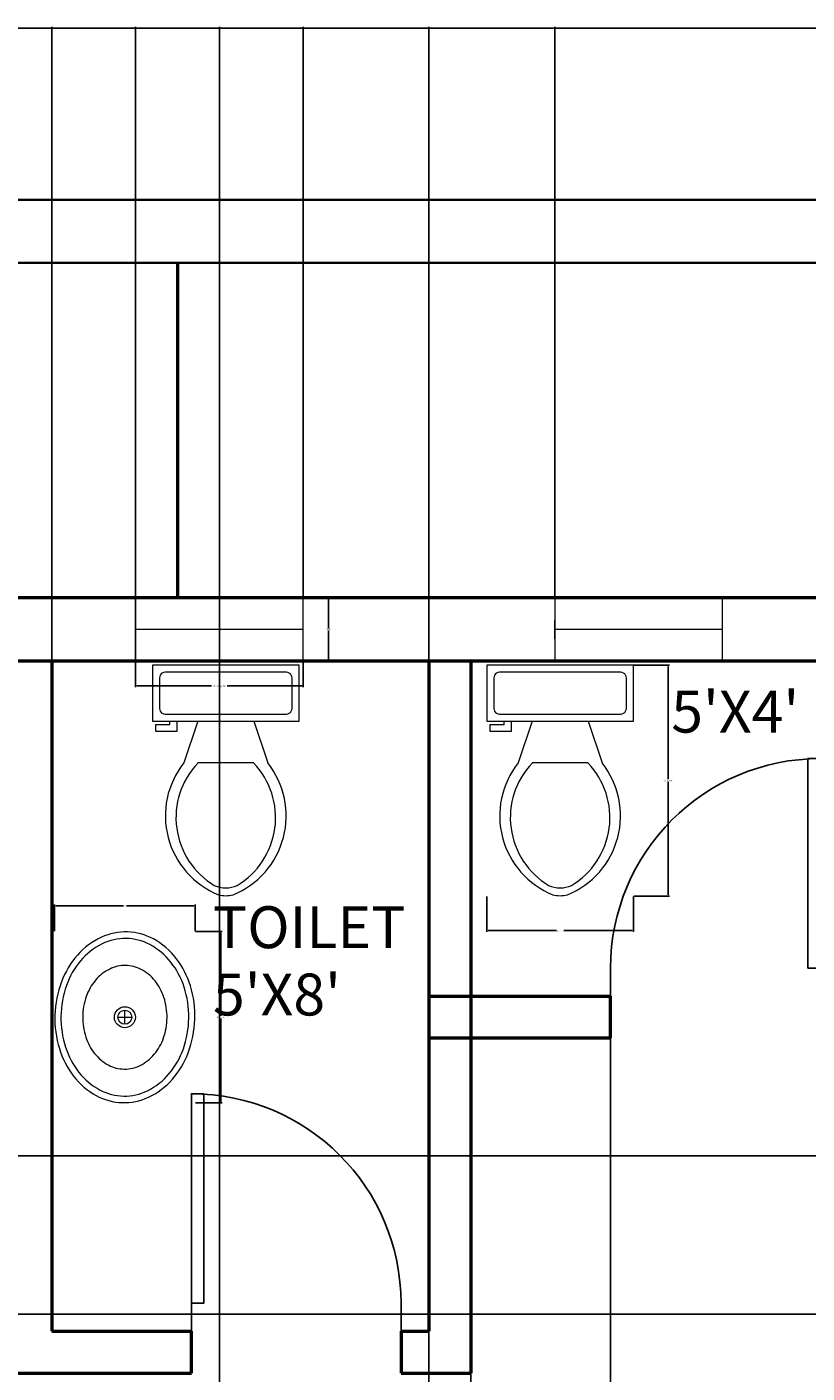
# Model space of a CAD drawing. Units: inches. Extents: x 8049 to 8459, y 820 to 1350.
# Tile 24 of 25: x 8182 to 8294, y 1157 to 1350. Entities that reach past the tile are written whole.
import ezdxf

# ---------------------------------------------------------------- set-up
doc = ezdxf.new("R2010")
doc.units = ezdxf.units.IN
doc.header["$MEASUREMENT"] = 0
for name, color, linetype, lineweight in [('A-ANNO-DIMS', 2, 'Continuous', 18), ('A-AREA-IDEN', 7, 'Continuous', 25), ('A-DOOR', 3, 'Continuous', 25), ('A-FLOR-FIXT', 9, 'Continuous', 18), ('A-GLAZ', 4, 'Continuous', 18), ('A-WALL', 7, 'Continuous', 50), ('C-SITE-WALL', 7, 'Continuous', 35)]:
    doc.layers.add(name, color=color, linetype=linetype, lineweight=lineweight)
doc.styles.get("Standard").update_dxf_attribs({"font": 'arial.ttf'})
doc.dimstyles.get("Standard").update_dxf_attribs({"dimtxt": 0.18, "dimasz": 0.18, "dimexe": 0.18, "dimexo": 0.0625, "dimgap": 0.09, "dimtad": 0, "dimtih": 1, "dimtoh": 1, "dimdec": 4, "dimzin": 0, "dimdsep": 46, "dimtxsty": 'Standard', "dimcen": 0.09, "dimadec": 0, "dimazin": 0, "dimtfac": 1, "dimtdec": 4, "dimtofl": 0, "dimtmove": 0, "dimatfit": 3, "dimfxl": 1, "dimtolj": 1, "dimtzin": 0, "dimarcsym": 0})

# ---------------------------------------------------------------- blocks, each defined once
blk = doc.blocks.new('*U2')
for p, q in [((0, 0), (0, -100)), ((750, 0), (750, -100))]:
    blk.add_line(p, q)
blk.add_lwpolyline([(0, 0), (0, 750), (43.75, 750), (43.75, 0)], close=True)
blk.add_arc((0, 0), 750, 0, 90)
blk = doc.blocks.new('*U4')
for p, q in [((0, 100), (0, 0)), ((900, 100), (900, 0)), ((0, 50), (900, 50))]:
    blk.add_line(p, q)
blk = doc.blocks.new('Sink - Oval top')
for p, q in [((-1, 0), (1, 0)), ((0, 1), (0, -1))]:
    blk.add_line(p, q)
for points in [[(-12.23, 0.39, 0.117634), (-11.46, -3.36, 0.104469), (-8.88, -6.8, 0.090016), (-5.08, -9.07, 0.08192), (-0.32, -10.02, 0.08192), (4.49, -9.38, 0.090016), (8.42, -7.36, 0.104469), (11.22, -4.09, 0.117634), (12.23, -0.39, 0.117634), (11.46, 3.36, 0.104469), (8.88, 6.8, 0.090016), (5.08, 9.07, 0.08192), (0.32, 10.02, 0.08192), (-4.49, 9.38, 0.090016), (-8.42, 7.36, 0.104469), (-11.22, 4.09, 0.117634)], [(-11.29, 0.16, 0.118622), (-10.52, -3.25, 0.104678), (-8.07, -6.36, 0.089562), (-4.54, -8.37, 0.081185), (-0.13, -9.15, 0.081185), (4.3, -8.49, 0.089562), (7.89, -6.58, 0.104678), (10.42, -3.55, 0.118622), (11.29, -0.16, 0.118622), (10.52, 3.25, 0.104678), (8.07, 6.36, 0.089562), (4.54, 8.37, 0.081185), (0.13, 9.15, 0.081185), (-4.3, 8.49, 0.089562), (-7.89, 6.58, 0.104678), (-10.42, 3.55, 0.118622)], [(-7.42, 0.08, 0.118283), (-6.91, -2.17, 0.104607), (-5.29, -4.21, 0.089718), (-2.97, -5.53, 0.081436), (-0.07, -6.04, 0.081436), (2.84, -5.59, 0.089718), (5.2, -4.33, 0.104607), (6.86, -2.32, 0.118283), (7.42, -0.08, 0.118283), (6.91, 2.17, 0.104607), (5.29, 4.21, 0.089718), (2.97, 5.53, 0.081436), (0.07, 6.04, 0.081436), (-2.84, 5.59, 0.089718), (-5.2, 4.33, 0.104607), (-6.86, 2.32, 0.118283)]]:
    blk.add_lwpolyline(points, format="xyb", close=True)
for radius in [1.5, 1]:
    blk.add_circle((0, 0), radius)
blk = doc.blocks.new('Toilet - top')
for p, q in [((9.5, -6), (9.5, -2)), ((-10, -8.5), (-8, -8.5)), ((-10, -9.5), (-10, -8.5)), ((-7, -9.5), (-10, -9.5)), ((-8, -8.5), (-8, -8)), ((-7, -8), (-7, -9.5)), ((-4, -8), (-6, -14)), ((4, -8), (6, -14)), ((4, -14), (-4, -14))]:
    blk.add_line(p, q)
blk.add_lwpolyline([(10.5, -8), (10.5, 0), (-10.5, 0), (-10.5, -8)], close=True)
for points in [[(8.5, -1), (-8.5, -1)], [(-9.5, -2), (-9.5, -6)], [(-8.5, -7), (8.5, -7)]]:
    blk.add_lwpolyline(points)
for centre, radius, start, end in [((-8.62, -1.88), 0.884, 81.8699, 188.1301), ((8.62, -1.88), 0.884, 351.8699, 98.1301), ((-8.62, -6.12), 0.884, 171.8699, 278.1301), ((8.62, -6.12), 0.884, 261.8699, 8.1301), ((3.52, -21.58), 12.17, 141.4691, 247.9714), ((4.2, -21.82), 11.33, 136.3677, 238.9468), ((-3.52, -21.58), 12.17, 292.0284, 38.5307), ((-4.2, -21.82), 11.33, 301.053, 43.6321), ((0, -27.88), 4, 245.7318, 294.2682), ((0, -29), 4, 254.8605, 285.1395)]:
    blk.add_arc(centre, radius, start, end)
blk = doc.blocks.new('WIN-24IN-SURROUND')
for p, q in [((24, 9), (0, 9)), ((0, 9), (0, 0)), ((24, 0), (24, 9))]:
    blk.add_line(p, q)
blk = doc.blocks.new('*D32')
at = {"layer": 'A-ANNO-DIMS', "color": 0, "lineweight": -2, "transparency": 16777216}
for p, q in [((8197.4, 1258.81), (8197.4, 1255.09)), ((8221.4, 1258.81), (8221.4, 1255.09)), ((8197.58, 1255.27), (8208.28, 1255.27)), ((8221.22, 1255.27), (8210.52, 1255.27))]:
    blk.add_line(p, q, dxfattribs=at)
at = {"layer": 'A-ANNO-DIMS', "color": 0, "transparency": 16777216}
for points in [[(8197.58, 1255.3), (8197.58, 1255.24), (8197.4, 1255.27)], [(8221.22, 1255.3), (8221.22, 1255.24), (8221.4, 1255.27)]]:
    blk.add_solid(points, dxfattribs=at)
at = {"layer": 'Defpoints', "color": 0, "transparency": 16777216}
for p in [(8197.4, 1258.87), (8221.4, 1258.87), (8221.4, 1255.27)]:
    blk.add_point(p, dxfattribs=at)
at = {"layer": 'A-ANNO-DIMS', "color": 0, "transparency": 16777216, "insert": (8209.4, 1255.27), "char_height": 0.18, "attachment_point": 5}
blk.add_mtext('\\A1;WINDOW 24 TYP.', dxfattribs=at)
blk = doc.blocks.new('*D33')
at = {"layer": 'A-ANNO-DIMS', "color": 0, "lineweight": -2, "transparency": 16777216}
for p, q in [((8221.46, 1267.87), (8225.18, 1267.87)), ((8225, 1267.69), (8225, 1263.55)), ((8225, 1259.05), (8225, 1263.19)), ((8221.46, 1258.87), (8225.18, 1258.87))]:
    blk.add_line(p, q, dxfattribs=at)
at = {"layer": 'A-ANNO-DIMS', "color": 0, "transparency": 16777216}
for points in [[(8224.97, 1267.69), (8225.03, 1267.69), (8225, 1267.87)], [(8224.97, 1259.05), (8225.03, 1259.05), (8225, 1258.87)]]:
    blk.add_solid(points, dxfattribs=at)
at = {"layer": 'Defpoints', "color": 0, "transparency": 16777216}
for p in [(8221.4, 1267.87), (8225, 1267.87), (8221.4, 1258.87)]:
    blk.add_point(p, dxfattribs=at)
at = {"layer": 'A-ANNO-DIMS', "color": 0, "transparency": 16777216, "insert": (8225, 1263.37), "char_height": 0.18, "attachment_point": 5}
blk.add_mtext('\\A1;9 TYP.', dxfattribs=at)
blk = doc.blocks.new('*D36')
at = {"layer": 'A-ANNO-DIMS', "color": 0, "lineweight": -2, "transparency": 16777216}
for p, q in [((8268.73, 1258.24), (8273.81, 1258.24)), ((8273.63, 1258.06), (8273.63, 1241.9)), ((8273.63, 1225.37), (8273.63, 1241.53)), ((8268.73, 1225.19), (8273.81, 1225.19))]:
    blk.add_line(p, q, dxfattribs=at)
at = {"layer": 'A-ANNO-DIMS', "color": 0, "transparency": 16777216}
for points in [[(8273.6, 1258.06), (8273.66, 1258.06), (8273.63, 1258.24)], [(8273.6, 1225.37), (8273.66, 1225.37), (8273.63, 1225.19)]]:
    blk.add_solid(points, dxfattribs=at)
at = {"layer": 'Defpoints', "color": 0, "transparency": 16777216}
for p in [(8268.67, 1258.24), (8273.63, 1258.24), (8268.67, 1225.19)]:
    blk.add_point(p, dxfattribs=at)
at = {"layer": 'A-ANNO-DIMS', "color": 0, "transparency": 16777216, "insert": (8273.63, 1241.72), "char_height": 0.18, "attachment_point": 5}
blk.add_mtext('\\A1;WC 33 TYP.', dxfattribs=at)
blk = doc.blocks.new('*D37')
at = {"layer": 'A-ANNO-DIMS', "color": 0, "lineweight": -2, "transparency": 16777216}
for p, q in [((8247.67, 1225.13), (8247.67, 1220.06)), ((8268.67, 1225.13), (8268.67, 1220.06)), ((8247.85, 1220.24), (8257.64, 1220.24)), ((8268.49, 1220.24), (8258.7, 1220.24))]:
    blk.add_line(p, q, dxfattribs=at)
at = {"layer": 'A-ANNO-DIMS', "color": 0, "transparency": 16777216}
for points in [[(8247.85, 1220.27), (8247.85, 1220.21), (8247.67, 1220.24)], [(8268.49, 1220.27), (8268.49, 1220.21), (8268.67, 1220.24)]]:
    blk.add_solid(points, dxfattribs=at)
at = {"layer": 'Defpoints', "color": 0, "transparency": 16777216}
for p in [(8247.67, 1225.19), (8268.67, 1225.19), (8268.67, 1220.24)]:
    blk.add_point(p, dxfattribs=at)
at = {"layer": 'A-ANNO-DIMS', "color": 0, "transparency": 16777216, "insert": (8258.17, 1220.24), "char_height": 0.18, "attachment_point": 5}
blk.add_mtext('\\A1;21 TYP.', dxfattribs=at)
blk = doc.blocks.new('*D44')
at = {"layer": 'A-ANNO-DIMS', "color": 0, "lineweight": -2, "transparency": 16777216}
for p, q in [((8205.99, 1220.1), (8209.79, 1220.1)), ((8209.61, 1219.92), (8209.61, 1208.01)), ((8209.61, 1195.73), (8209.61, 1207.64)), ((8205.99, 1195.55), (8209.79, 1195.55))]:
    blk.add_line(p, q, dxfattribs=at)
at = {"layer": 'A-ANNO-DIMS', "color": 0, "transparency": 16777216}
for points in [[(8209.58, 1219.92), (8209.64, 1219.92), (8209.61, 1220.1)], [(8209.58, 1195.73), (8209.64, 1195.73), (8209.61, 1195.55)]]:
    blk.add_solid(points, dxfattribs=at)
at = {"layer": 'Defpoints', "color": 0, "transparency": 16777216}
for p in [(8205.93, 1220.1), (8209.61, 1220.1), (8205.93, 1195.55)]:
    blk.add_point(p, dxfattribs=at)
at = {"layer": 'A-ANNO-DIMS', "color": 0, "transparency": 16777216, "insert": (8209.61, 1207.83), "char_height": 0.18, "attachment_point": 5}
blk.add_mtext('\\A1;BASIN 25', dxfattribs=at)
blk = doc.blocks.new('*D45')
at = {"layer": 'A-ANNO-DIMS', "color": 0, "lineweight": -2, "transparency": 16777216}
for p, q in [((8185.79, 1220.17), (8185.79, 1223.97)), ((8185.97, 1223.79), (8195.64, 1223.79)), ((8205.75, 1223.79), (8196.08, 1223.79)), ((8205.93, 1220.17), (8205.93, 1223.97))]:
    blk.add_line(p, q, dxfattribs=at)
at = {"layer": 'A-ANNO-DIMS', "color": 0, "transparency": 16777216}
for points in [[(8185.97, 1223.82), (8185.97, 1223.76), (8185.79, 1223.79)], [(8205.75, 1223.82), (8205.75, 1223.76), (8205.93, 1223.79)]]:
    blk.add_solid(points, dxfattribs=at)
at = {"layer": 'Defpoints', "color": 0, "transparency": 16777216}
for p in [(8185.79, 1223.79), (8185.79, 1220.1), (8205.93, 1220.1)]:
    blk.add_point(p, dxfattribs=at)
at = {"layer": 'A-ANNO-DIMS', "color": 0, "transparency": 16777216, "insert": (8195.86, 1223.79), "char_height": 0.18, "attachment_point": 5}
blk.add_mtext('\\A1;20', dxfattribs=at)
blk = doc.blocks.new('*D48')
at = {"layer": 'A-ANNO-DIMS', "color": 0, "lineweight": -2, "transparency": 16777216}
for p, q in [((8074.4, 1324.93), (8074.4, 1349.65)), ((8074.58, 1349.47), (8254.11, 1349.47)), ((8434.22, 1349.47), (8254.69, 1349.47)), ((8434.4, 1324.93), (8434.4, 1349.65))]:
    blk.add_line(p, q, dxfattribs=at)
at = {"layer": 'A-ANNO-DIMS', "color": 0, "transparency": 16777216}
for points in [[(8074.58, 1349.5), (8074.58, 1349.44), (8074.4, 1349.47)], [(8434.22, 1349.5), (8434.22, 1349.44), (8434.4, 1349.47)]]:
    blk.add_solid(points, dxfattribs=at)
at = {"layer": 'Defpoints', "color": 0, "transparency": 16777216}
for p in [(8434.4, 1349.47), (8074.4, 1324.87), (8434.4, 1324.87)]:
    blk.add_point(p, dxfattribs=at)
at = {"layer": 'A-ANNO-DIMS', "color": 0, "transparency": 16777216, "insert": (8254.4, 1349.47), "char_height": 0.18, "attachment_point": 5}
blk.add_mtext('\\A1;360', dxfattribs=at)
blk = doc.blocks.new('*D64')
at = {"layer": 'A-ANNO-DIMS', "color": 0, "lineweight": -2, "transparency": 16777216}
for p, q in [((8185.4, 1258.93), (8185.4, 1349.65)), ((8185.58, 1349.47), (8191.19, 1349.47)), ((8197.22, 1349.47), (8191.61, 1349.47)), ((8197.4, 1258.93), (8197.4, 1349.65))]:
    blk.add_line(p, q, dxfattribs=at)
at = {"layer": 'A-ANNO-DIMS', "color": 0, "transparency": 16777216}
for points in [[(8185.58, 1349.5), (8185.58, 1349.44), (8185.4, 1349.47)], [(8197.22, 1349.5), (8197.22, 1349.44), (8197.4, 1349.47)]]:
    blk.add_solid(points, dxfattribs=at)
at = {"layer": 'Defpoints', "color": 0, "transparency": 16777216}
for p in [(8185.4, 1349.47), (8185.4, 1258.87), (8197.4, 1258.87)]:
    blk.add_point(p, dxfattribs=at)
at = {"layer": 'A-ANNO-DIMS', "color": 0, "transparency": 16777216, "insert": (8191.4, 1349.47), "char_height": 0.18, "attachment_point": 5}
blk.add_mtext('\\A1;12', dxfattribs=at)
blk = doc.blocks.new('*D65')
at = {"layer": 'A-ANNO-DIMS', "color": 0, "lineweight": -2, "transparency": 16777216}
for p, q in [((8221.4, 1267.93), (8221.4, 1349.65)), ((8221.58, 1349.47), (8239.18, 1349.47)), ((8257.22, 1349.47), (8239.62, 1349.47)), ((8257.4, 1267.93), (8257.4, 1349.65))]:
    blk.add_line(p, q, dxfattribs=at)
at = {"layer": 'A-ANNO-DIMS', "color": 0, "transparency": 16777216}
for points in [[(8221.58, 1349.5), (8221.58, 1349.44), (8221.4, 1349.47)], [(8257.22, 1349.5), (8257.22, 1349.44), (8257.4, 1349.47)]]:
    blk.add_solid(points, dxfattribs=at)
at = {"layer": 'Defpoints', "color": 0, "transparency": 16777216}
for p in [(8257.4, 1349.47), (8221.4, 1267.87), (8257.4, 1267.87)]:
    blk.add_point(p, dxfattribs=at)
at = {"layer": 'A-ANNO-DIMS', "color": 0, "transparency": 16777216, "insert": (8239.4, 1349.47), "char_height": 0.18, "attachment_point": 5}
blk.add_mtext('\\A1;36', dxfattribs=at)
blk = doc.blocks.new('*D73')
at = {"layer": 'A-ANNO-DIMS', "color": 0, "lineweight": -2, "transparency": 16777216}
for p, q in [((8239.4, 1204.81), (8239.4, 820.09)), ((8265.4, 1204.81), (8265.4, 820.09)), ((8239.58, 820.27), (8252.18, 820.27)), ((8265.22, 820.27), (8252.62, 820.27))]:
    blk.add_line(p, q, dxfattribs=at)
at = {"layer": 'A-ANNO-DIMS', "color": 0, "transparency": 16777216}
for points in [[(8239.58, 820.3), (8239.58, 820.24), (8239.4, 820.27)], [(8265.22, 820.3), (8265.22, 820.24), (8265.4, 820.27)]]:
    blk.add_solid(points, dxfattribs=at)
at = {"layer": 'Defpoints', "color": 0, "transparency": 16777216}
for p in [(8239.4, 1204.87), (8265.4, 1204.87), (8265.4, 820.27)]:
    blk.add_point(p, dxfattribs=at)
at = {"layer": 'A-ANNO-DIMS', "color": 0, "transparency": 16777216, "insert": (8252.4, 820.27), "char_height": 0.18, "attachment_point": 5}
blk.add_mtext('\\A1;26', dxfattribs=at)
blk = doc.blocks.new('*D75')
at = {"layer": 'A-ANNO-DIMS', "color": 0, "lineweight": -2, "transparency": 16777216}
for p, q in [((8239.4, 1162.81), (8239.4, 820.09)), ((8245.4, 1156.81), (8245.4, 820.09)), ((8239.58, 820.27), (8242.25, 820.27)), ((8245.22, 820.27), (8242.55, 820.27))]:
    blk.add_line(p, q, dxfattribs=at)
at = {"layer": 'A-ANNO-DIMS', "color": 0, "transparency": 16777216}
for points in [[(8239.58, 820.3), (8239.58, 820.24), (8239.4, 820.27)], [(8245.22, 820.3), (8245.22, 820.24), (8245.4, 820.27)]]:
    blk.add_solid(points, dxfattribs=at)
at = {"layer": 'Defpoints', "color": 0, "transparency": 16777216}
for p in [(8239.4, 1162.87), (8245.4, 1156.87), (8245.4, 820.27)]:
    blk.add_point(p, dxfattribs=at)
at = {"layer": 'A-ANNO-DIMS', "color": 0, "transparency": 16777216, "insert": (8242.4, 820.27), "char_height": 0.18, "attachment_point": 5}
blk.add_mtext('\\A1;6', dxfattribs=at)
blk = doc.blocks.new('*D79')
at = {"layer": 'A-ANNO-DIMS', "color": 0, "lineweight": -2, "transparency": 16777216}
for p, q in [((8157.59, 1082.57), (8157.59, 1349.65)), ((8157.77, 1349.47), (8183.11, 1349.47)), ((8209.23, 1349.47), (8183.9, 1349.47)), ((8209.41, 1082.57), (8209.41, 1349.65))]:
    blk.add_line(p, q, dxfattribs=at)
at = {"layer": 'A-ANNO-DIMS', "color": 0, "transparency": 16777216}
for points in [[(8157.77, 1349.5), (8157.77, 1349.44), (8157.59, 1349.47)], [(8209.23, 1349.5), (8209.23, 1349.44), (8209.41, 1349.47)]]:
    blk.add_solid(points, dxfattribs=at)
at = {"layer": 'Defpoints', "color": 0, "transparency": 16777216}
for p in [(8209.41, 1349.47), (8157.59, 1082.51), (8209.41, 1082.51)]:
    blk.add_point(p, dxfattribs=at)
at = {"layer": 'A-ANNO-DIMS', "color": 0, "transparency": 16777216, "insert": (8183.5, 1349.47), "char_height": 0.18, "attachment_point": 5}
blk.add_mtext('\\A1;51.82', dxfattribs=at)
blk = doc.blocks.new('*D83')
at = {"layer": 'A-ANNO-DIMS', "color": 0, "lineweight": -2, "transparency": 16777216}
for p, q in [((8112.96, 1187.99), (8459.18, 1187.99)), ((8459, 1187.81), (8459, 1176.83)), ((8459, 1165.49), (8459, 1176.47)), ((8112.96, 1165.31), (8459.18, 1165.31))]:
    blk.add_line(p, q, dxfattribs=at)
at = {"layer": 'A-ANNO-DIMS', "color": 0, "transparency": 16777216}
for points in [[(8458.97, 1187.81), (8459.03, 1187.81), (8459, 1187.99)], [(8458.97, 1165.49), (8459.03, 1165.49), (8459, 1165.31)]]:
    blk.add_solid(points, dxfattribs=at)
at = {"layer": 'Defpoints', "color": 0, "transparency": 16777216}
for p in [(8112.9, 1187.99), (8459, 1187.99), (8112.9, 1165.31)]:
    blk.add_point(p, dxfattribs=at)
at = {"layer": 'A-ANNO-DIMS', "color": 0, "transparency": 16777216, "insert": (8459, 1176.65), "char_height": 0.18, "attachment_point": 5}
blk.add_mtext('\\A1;22.68', dxfattribs=at)
blk = doc.blocks.new('*D86')
at = {"layer": 'A-ANNO-DIMS', "color": 0, "lineweight": -2, "transparency": 16777216}
for p, q in [((8265.4, 1204.81), (8265.4, 820.09)), ((8295.4, 1204.81), (8295.4, 820.09)), ((8265.58, 820.27), (8280.18, 820.27)), ((8295.22, 820.27), (8280.62, 820.27))]:
    blk.add_line(p, q, dxfattribs=at)
at = {"layer": 'A-ANNO-DIMS', "color": 0, "transparency": 16777216}
for points in [[(8265.58, 820.3), (8265.58, 820.24), (8265.4, 820.27)], [(8295.22, 820.3), (8295.22, 820.24), (8295.4, 820.27)]]:
    blk.add_solid(points, dxfattribs=at)
at = {"layer": 'Defpoints', "color": 0, "transparency": 16777216}
for p in [(8265.4, 1204.87), (8295.4, 1204.87), (8295.4, 820.27)]:
    blk.add_point(p, dxfattribs=at)
at = {"layer": 'A-ANNO-DIMS', "color": 0, "transparency": 16777216, "insert": (8280.4, 820.27), "char_height": 0.18, "attachment_point": 5}
blk.add_mtext('\\A1;30', dxfattribs=at)
blk = doc.blocks.new('*D87')
at = {"layer": 'A-ANNO-DIMS', "color": 0, "lineweight": -2, "transparency": 16777216}
for p, q in [((8185.4, 1258.93), (8185.4, 1349.65)), ((8185.58, 1349.47), (8212.18, 1349.47)), ((8239.22, 1349.47), (8212.62, 1349.47)), ((8239.4, 1258.93), (8239.4, 1349.65))]:
    blk.add_line(p, q, dxfattribs=at)
at = {"layer": 'A-ANNO-DIMS', "color": 0, "transparency": 16777216}
for points in [[(8185.58, 1349.5), (8185.58, 1349.44), (8185.4, 1349.47)], [(8239.22, 1349.5), (8239.22, 1349.44), (8239.4, 1349.47)]]:
    blk.add_solid(points, dxfattribs=at)
at = {"layer": 'Defpoints', "color": 0, "transparency": 16777216}
for p in [(8239.4, 1349.47), (8185.4, 1258.87), (8239.4, 1258.87)]:
    blk.add_point(p, dxfattribs=at)
at = {"layer": 'A-ANNO-DIMS', "color": 0, "transparency": 16777216, "insert": (8212.4, 1349.47), "char_height": 0.18, "attachment_point": 5}
blk.add_mtext('\\A1;54', dxfattribs=at)

msp = doc.modelspace()

# ---------------------------------------------------------------- linework, layer by layer
at = {"layer": 'A-WALL'}
for p, q in [((8203.3974, 1315.8706), (8203.3974, 1267.8706)), ((8425.3974, 1267.8706), (8117.3974, 1267.8706)), ((8117.3974, 1258.8706), (8425.3974, 1258.8706)), ((8185.3974, 1258.8706), (8185.3974, 1162.8706)), ((8239.3974, 1258.8706), (8239.3974, 1162.8706)), ((8245.3974, 1258.8706), (8245.3974, 1156.8706)), ((8239.3974, 1210.8706), (8265.3974, 1210.8706)), ((8265.3974, 1204.8706), (8265.3974, 1210.8706)), ((8239.3974, 1204.8706), (8265.3974, 1204.8706)), ((8185.3974, 1162.8706), (8205.3974, 1162.8706)), ((8205.3974, 1156.8706), (8205.3974, 1162.8706)), ((8235.3974, 1162.8706), (8235.3974, 1156.8706)), ((8235.3974, 1162.8706), (8239.3974, 1162.8706)), ((8175.3974, 1156.8706), (8205.3974, 1156.8706)), ((8235.3974, 1156.8706), (8245.3974, 1156.8706))]:
    msp.add_line(p, q, dxfattribs=at)
at = {"layer": 'C-SITE-WALL'}
for p, q in [((8434.3974, 1324.8706), (8074.3974, 1324.8706)), ((8425.3974, 1315.8706), (8083.3974, 1315.8706))]:
    msp.add_line(p, q, dxfattribs=at)

# ---------------------------------------------------------------- block references
at = {"layer": 'A-DOOR', "yscale": 0.0399999999999999, "zscale": 0.0399999999999999}
for p, xscale in [((8295.3974, 1214.8706), -0.0399999999999999), ((8205.3974, 1166.8706), 0.0399999999999999)]:
    msp.add_blockref('*U2', p, dxfattribs=dict(at, xscale=xscale))
at = {"layer": 'A-FLOR-FIXT'}
for p in [(8210.306, 1258.239), (8258.1718, 1258.239)]:
    msp.add_blockref('Toilet - top', p, dxfattribs=at)
at = {"layer": 'A-FLOR-FIXT', "rotation": 90}
msp.add_blockref('Sink - Oval top', (8195.8603, 1207.8275), dxfattribs=at)
at = {"layer": 'A-GLAZ'}
for p in [(8197.397, 1258.871), (8257.397, 1258.871)]:
    msp.add_blockref('WIN-24IN-SURROUND', p, dxfattribs=at)
at = {"layer": 'A-GLAZ', "xscale": 0.0266666666666666, "yscale": 0.0266666666666666, "zscale": 0.0266666666666666, "rotation": 180}
for p in [(8221.3974, 1264.7039), (8281.3974, 1264.7039)]:
    msp.add_blockref('*U4', p, dxfattribs=at)

# ---------------------------------------------------------------- texts
at = {"layer": 'A-AREA-IDEN'}
for s, p in [("5'X4'", (8274.0826, 1248.5983)), ('TOILET', (8208.4759, 1217.722)), ("5'X8'", (8208.4759, 1208.0835))]:
    msp.add_text(s, height=6, dxfattribs=at).set_placement(p)

# ---------------------------------------------------------------- dimensions: what is measured, and where the dimension line sits
at = {"layer": 'A-ANNO-DIMS'}
for base, p1, p2, override, picture, middle in [((8434.3974, 1349.4706), (8074.3974, 1324.8706), (8434.3974, 1324.8706), {"dimdec": 0, "dimlfac": 1, "dimrnd": 0, "dimzin": 0, "dimdsep": 46, "dimlunit": 2}, '*D48', (8254.3974, 1349.4706)), ((8209.4146, 1349.4706), (8157.5937, 1082.5119), (8209.4146, 1082.5119), {"dimdec": 2, "dimlfac": 1, "dimrnd": 0, "dimzin": 0, "dimdsep": 46, "dimlunit": 2}, '*D79', (8183.5041, 1349.4706)), ((8185.3974, 1349.4706), (8197.3974, 1258.8706), (8185.3974, 1258.8706), {"dimdec": 0, "dimlfac": 1, "dimrnd": 0, "dimzin": 0, "dimdsep": 46, "dimlunit": 2}, '*D64', (8191.3974, 1349.4706)), ((8239.3974, 1349.4706), (8185.3974, 1258.8706), (8239.3974, 1258.8706), {"dimdec": 0, "dimlfac": 1, "dimrnd": 0, "dimzin": 0, "dimdsep": 46, "dimlunit": 2}, '*D87', (8212.3974, 1349.4706)), ((8257.3974, 1349.4706), (8221.3974, 1267.8706), (8257.3974, 1267.8706), {"dimdec": 0, "dimlfac": 1, "dimrnd": 0, "dimzin": 0, "dimdsep": 46, "dimlunit": 2}, '*D65', (8239.3974, 1349.4706)), ((8265.3974, 820.2706), (8239.3974, 1204.8706), (8265.3974, 1204.8706), {"dimdec": 0, "dimlfac": 1, "dimrnd": 0, "dimzin": 0, "dimdsep": 46, "dimlunit": 2}, '*D73', (8252.3974, 820.2706)), ((8295.3974, 820.2706), (8265.3974, 1204.8706), (8295.3974, 1204.8706), {"dimdec": 0, "dimlfac": 1, "dimrnd": 0, "dimzin": 0, "dimdsep": 46, "dimlunit": 2}, '*D86', (8280.3974, 820.2706)), ((8245.3974, 820.2706), (8239.3974, 1162.8706), (8245.3974, 1156.8706), {"dimdec": 0, "dimlfac": 1, "dimrnd": 0, "dimzin": 0, "dimdsep": 46, "dimlunit": 2}, '*D75', (8242.3974, 820.2706))]:
    dim = msp.add_linear_dim(base=base, p1=p1, p2=p2, dimstyle='Standard', override=override, dxfattribs=at)
    dim.commit()
    dim.dimension.update_dxf_attribs({"geometry": picture, "text_midpoint": middle})
for base, p1, p2, text, picture, middle in [((8224.9974, 1267.8706), (8221.3974, 1258.8706), (8221.3974, 1267.8706), '<> TYP.', '*D33', (8224.9974, 1263.3706)), ((8273.6288, 1258.239), (8268.6718, 1225.1927), (8268.6718, 1258.239), 'WC <> TYP.', '*D36', (8273.6288, 1241.7158)), ((8209.6112, 1220.1029), (8205.9286, 1195.552), (8205.9286, 1220.1029), 'BASIN <>', '*D44', (8209.6112, 1207.8275))]:
    dim = msp.add_linear_dim(base=base, p1=p1, p2=p2, angle=90, text=text, dimstyle='Standard', override={"dimdec": 0, "dimlfac": 1, "dimrnd": 0, "dimzin": 0, "dimdsep": 46, "dimlunit": 2}, dxfattribs=at)
    dim.commit()
    dim.dimension.update_dxf_attribs({"geometry": picture, "text_midpoint": middle})
for base, p1, p2, text, picture, middle in [((8221.3974, 1255.2706), (8197.3974, 1258.8706), (8221.3974, 1258.8706), 'WINDOW <> TYP.', '*D32', (8209.3974, 1255.2706)), ((8268.6718, 1220.2358), (8247.6718, 1225.1927), (8268.6718, 1225.1927), '<> TYP.', '*D37', (8258.1718, 1220.2358))]:
    dim = msp.add_linear_dim(base=base, p1=p1, p2=p2, text=text, dimstyle='Standard', override={"dimdec": 0, "dimlfac": 1, "dimrnd": 0, "dimzin": 0, "dimdsep": 46, "dimlunit": 2}, dxfattribs=at)
    dim.commit()
    dim.dimension.update_dxf_attribs({"geometry": picture, "text_midpoint": middle})
for base, p1, p2, angle, override, picture, middle in [((8185.792, 1223.7855), (8205.9286, 1220.1029), (8185.792, 1220.1029), 180, {"dimdec": 0, "dimlfac": 1, "dimrnd": 0, "dimzin": 0, "dimdsep": 46, "dimlunit": 2}, '*D45', (8195.8603, 1223.7855)), ((8458.9974, 1187.9939), (8112.9001, 1165.3117), (8112.9001, 1187.9939), 90, {"dimdec": 2, "dimlfac": 1, "dimrnd": 0, "dimzin": 0, "dimdsep": 46, "dimlunit": 2}, '*D83', (8458.9974, 1176.6528))]:
    dim = msp.add_linear_dim(base=base, p1=p1, p2=p2, angle=angle, dimstyle='Standard', override=override, dxfattribs=at)
    dim.commit()
    dim.dimension.update_dxf_attribs({"geometry": picture, "text_midpoint": middle})

doc.saveas('drawing.dxf')
